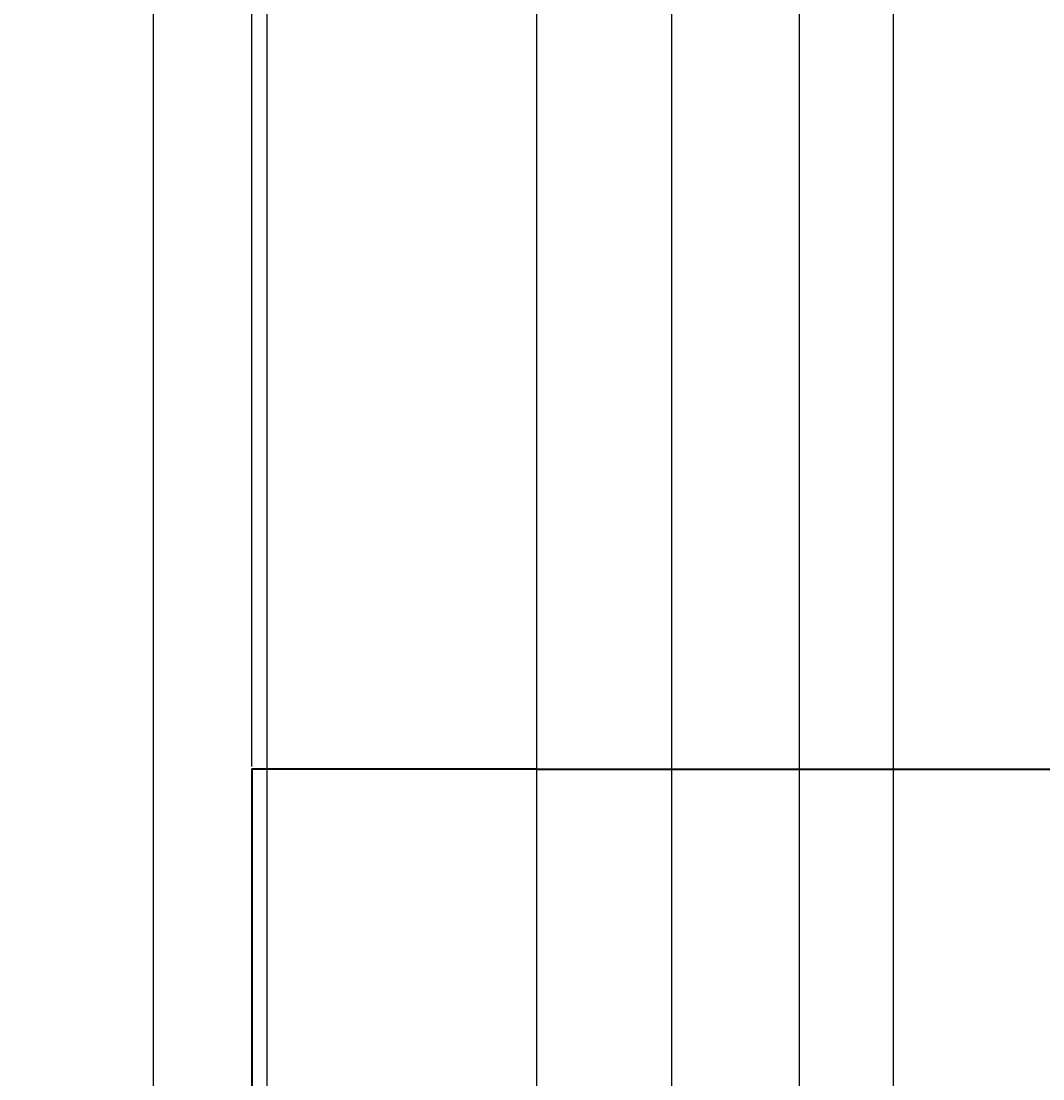
# Model space of a CAD drawing. Units: inches. Extents: x -6 to 289, y -8 to 323.
# Tile 79 of 107: x 104 to 126, y 252 to 276. Entities that reach past the tile are written whole.
import ezdxf

# ---------------------------------------------------------------- set-up
doc = ezdxf.new("R2010")
doc.units = ezdxf.units.IN
doc.header["$MEASUREMENT"] = 0
doc.layers.add('A-ANNO-DIMS', color=2, linetype='Continuous', lineweight=18)
doc.layers.add('A-ELEV', color=7, linetype='Continuous', lineweight=35)
doc.styles.get("Standard").update_dxf_attribs({"font": 'arial.ttf'})
doc.dimstyles.get("Standard").update_dxf_attribs({"dimtxt": 0.18, "dimasz": 0.18, "dimexe": 0.18, "dimexo": 0.0625, "dimgap": 0.09, "dimtad": 0, "dimtih": 1, "dimtoh": 1, "dimdec": 4, "dimzin": 0, "dimdsep": 46, "dimtxsty": 'Standard', "dimcen": 0.09, "dimadec": 0, "dimazin": 0, "dimtfac": 1, "dimtdec": 4, "dimtofl": 0, "dimtmove": 0, "dimatfit": 3, "dimfxl": 1, "dimtolj": 1, "dimtzin": 0, "dimarcsym": 0})

# ---------------------------------------------------------------- blocks, each defined once
blk = doc.blocks.new('*D10')
at = {"layer": 'A-ANNO-DIMS', "color": 0, "lineweight": -2, "transparency": 16777216}
for p, q in [((115.164, 307.351), (115.164, 322.969)), ((126.883, 226.717), (126.883, 322.969)), ((115.344, 322.789), (120.639, 322.789)), ((126.703, 322.789), (121.408, 322.789))]:
    blk.add_line(p, q, dxfattribs=at)
at = {"layer": 'A-ANNO-DIMS', "color": 0, "transparency": 16777216}
for points in [[(115.344, 322.819), (115.344, 322.759), (115.164, 322.789)], [(126.703, 322.819), (126.703, 322.759), (126.883, 322.789)]]:
    blk.add_solid(points, dxfattribs=at)
at = {"layer": 'Defpoints', "color": 0, "transparency": 16777216}
for p in [(126.883, 322.789), (115.164, 307.289), (126.883, 226.654)]:
    blk.add_point(p, dxfattribs=at)
at = {"layer": 'A-ANNO-DIMS', "color": 0, "transparency": 16777216, "insert": (121.024, 322.789), "char_height": 0.18, "attachment_point": 5}
blk.add_mtext('\\A1;11.72', dxfattribs=at)
blk = doc.blocks.new('*D27')
at = {"layer": 'A-ANNO-DIMS', "color": 0, "lineweight": -2, "transparency": 16777216}
for p, q in [((19.226, 307.289), (288.653, 307.289)), ((288.473, 307.109), (288.473, 277.471)), ((288.473, 247.469), (288.473, 277.107)), ((247.226, 247.289), (288.653, 247.289))]:
    blk.add_line(p, q, dxfattribs=at)
at = {"layer": 'A-ANNO-DIMS', "color": 0, "transparency": 16777216}
for points in [[(288.443, 307.109), (288.503, 307.109), (288.473, 307.289)], [(288.443, 247.469), (288.503, 247.469), (288.473, 247.289)]]:
    blk.add_solid(points, dxfattribs=at)
at = {"layer": 'Defpoints', "color": 0, "transparency": 16777216}
for p in [(19.164, 307.289), (288.473, 307.289), (247.164, 247.289)]:
    blk.add_point(p, dxfattribs=at)
at = {"layer": 'A-ANNO-DIMS', "color": 0, "transparency": 16777216, "insert": (288.473, 277.289), "char_height": 0.18, "attachment_point": 5}
blk.add_mtext('\\A1;60', dxfattribs=at)
blk = doc.blocks.new('*D58')
at = {"layer": 'A-ANNO-DIMS', "color": 0, "lineweight": -2, "transparency": 16777216}
for p, q in [((106.634, 68.495), (106.634, 322.969)), ((123.094, 68.495), (123.094, 322.969)), ((106.814, 322.789), (114.479, 322.789)), ((122.914, 322.789), (115.249, 322.789))]:
    blk.add_line(p, q, dxfattribs=at)
at = {"layer": 'A-ANNO-DIMS', "color": 0, "transparency": 16777216}
for points in [[(106.814, 322.819), (106.814, 322.759), (106.634, 322.789)], [(122.914, 322.819), (122.914, 322.759), (123.094, 322.789)]]:
    blk.add_solid(points, dxfattribs=at)
at = {"layer": 'Defpoints', "color": 0, "transparency": 16777216}
for p in [(123.094, 322.789), (106.634, 68.432), (123.094, 68.432)]:
    blk.add_point(p, dxfattribs=at)
at = {"layer": 'A-ANNO-DIMS', "color": 0, "transparency": 16777216, "insert": (114.864, 322.789), "char_height": 0.18, "attachment_point": 5}
blk.add_mtext('\\A1;16.46', dxfattribs=at)
blk = doc.blocks.new('*D73')
at = {"layer": 'A-ANNO-DIMS', "color": 0, "lineweight": -2, "transparency": 16777216}
for p, q in [((121.008, 51.148), (121.008, 322.969)), ((135.296, 51.148), (135.296, 322.969)), ((121.188, 322.789), (127.697, 322.789)), ((135.116, 322.789), (128.607, 322.789))]:
    blk.add_line(p, q, dxfattribs=at)
at = {"layer": 'A-ANNO-DIMS', "color": 0, "transparency": 16777216}
for points in [[(121.188, 322.819), (121.188, 322.759), (121.008, 322.789)], [(135.116, 322.819), (135.116, 322.759), (135.296, 322.789)]]:
    blk.add_solid(points, dxfattribs=at)
at = {"layer": 'Defpoints', "color": 0, "transparency": 16777216}
for p in [(135.296, 322.789), (121.008, 51.085), (135.296, 51.085)]:
    blk.add_point(p, dxfattribs=at)
at = {"layer": 'A-ANNO-DIMS', "color": 0, "transparency": 16777216, "insert": (128.152, 322.789), "char_height": 0.18, "attachment_point": 5}
blk.add_mtext('\\A1;14.288', dxfattribs=at)
blk = doc.blocks.new('*D92')
at = {"layer": 'A-ANNO-DIMS', "color": 0, "lineweight": -2, "transparency": 16777216}
for p, q in [((109.164, 127.351), (109.164, 322.969)), ((115.164, 162.411), (115.164, 322.969)), ((109.344, 322.789), (112.014, 322.789)), ((114.984, 322.789), (112.313, 322.789))]:
    blk.add_line(p, q, dxfattribs=at)
at = {"layer": 'A-ANNO-DIMS', "color": 0, "transparency": 16777216}
for points in [[(109.344, 322.819), (109.344, 322.759), (109.164, 322.789)], [(114.984, 322.819), (114.984, 322.759), (115.164, 322.789)]]:
    blk.add_solid(points, dxfattribs=at)
at = {"layer": 'Defpoints', "color": 0, "transparency": 16777216}
for p in [(115.164, 322.789), (115.164, 162.348), (109.164, 127.289)]:
    blk.add_point(p, dxfattribs=at)
at = {"layer": 'A-ANNO-DIMS', "color": 0, "transparency": 16777216, "insert": (112.164, 322.789), "char_height": 0.18, "attachment_point": 5}
blk.add_mtext('\\A1;6', dxfattribs=at)
blk = doc.blocks.new('*D93')
at = {"layer": 'A-ANNO-DIMS', "color": 0, "lineweight": -2, "transparency": 16777216}
for p, q in [((115.164, 162.411), (115.164, 322.969)), ((118.164, 159.411), (118.164, 322.969)), ((115.344, 322.789), (116.515, 322.789)), ((117.984, 322.789), (116.813, 322.789))]:
    blk.add_line(p, q, dxfattribs=at)
at = {"layer": 'A-ANNO-DIMS', "color": 0, "transparency": 16777216}
for points in [[(115.344, 322.819), (115.344, 322.759), (115.164, 322.789)], [(117.984, 322.819), (117.984, 322.759), (118.164, 322.789)]]:
    blk.add_solid(points, dxfattribs=at)
at = {"layer": 'Defpoints', "color": 0, "transparency": 16777216}
for p in [(118.164, 322.789), (115.164, 162.348), (118.164, 159.348)]:
    blk.add_point(p, dxfattribs=at)
at = {"layer": 'A-ANNO-DIMS', "color": 0, "transparency": 16777216, "insert": (116.664, 322.789), "char_height": 0.18, "attachment_point": 5}
blk.add_mtext('\\A1;3', dxfattribs=at)
blk = doc.blocks.new('*D94')
at = {"layer": 'A-ANNO-DIMS', "color": 0, "lineweight": -2, "transparency": 16777216}
for p, q in [((118.164, 159.411), (118.164, 322.969)), ((161.552, 159.411), (161.552, 322.969)), ((118.344, 322.789), (139.46, 322.789)), ((161.372, 322.789), (140.256, 322.789))]:
    blk.add_line(p, q, dxfattribs=at)
at = {"layer": 'A-ANNO-DIMS', "color": 0, "transparency": 16777216}
for points in [[(118.344, 322.819), (118.344, 322.759), (118.164, 322.789)], [(161.372, 322.819), (161.372, 322.759), (161.552, 322.789)]]:
    blk.add_solid(points, dxfattribs=at)
at = {"layer": 'Defpoints', "color": 0, "transparency": 16777216}
for p in [(161.552, 322.789), (118.164, 159.348), (161.552, 159.348)]:
    blk.add_point(p, dxfattribs=at)
at = {"layer": 'A-ANNO-DIMS', "color": 0, "transparency": 16777216, "insert": (139.858, 322.789), "char_height": 0.18, "attachment_point": 5}
blk.add_mtext('\\A1;43.39', dxfattribs=at)
blk = doc.blocks.new('*D105')
at = {"layer": 'A-ANNO-DIMS', "color": 0, "lineweight": -2, "transparency": 16777216}
for p, q in [((108.823, 259.351), (108.823, 322.969)), ((115.164, 277.105), (115.164, 322.969)), ((109.003, 322.789), (111.616, 322.789)), ((114.984, 322.789), (112.37, 322.789))]:
    blk.add_line(p, q, dxfattribs=at)
at = {"layer": 'A-ANNO-DIMS', "color": 0, "transparency": 16777216}
for points in [[(109.003, 322.819), (109.003, 322.759), (108.823, 322.789)], [(114.984, 322.819), (114.984, 322.759), (115.164, 322.789)]]:
    blk.add_solid(points, dxfattribs=at)
at = {"layer": 'Defpoints', "color": 0, "transparency": 16777216}
for p in [(115.164, 322.789), (115.164, 277.043), (108.823, 259.289)]:
    blk.add_point(p, dxfattribs=at)
at = {"layer": 'A-ANNO-DIMS', "color": 0, "transparency": 16777216, "insert": (111.993, 322.789), "char_height": 0.18, "attachment_point": 5}
blk.add_mtext('\\A1;6.341', dxfattribs=at)

msp = doc.modelspace()

# ---------------------------------------------------------------- linework, layer by layer
at = {"layer": 'A-ELEV'}
msp.add_line((115.1638, 259.2888), (271.1638, 259.2888), dxfattribs=at)
msp.add_lwpolyline([(115.1638, 259.2888), (108.8227, 259.2888), (108.8227, 247.2888), (115.1638, 247.2888)], dxfattribs=at)

# ---------------------------------------------------------------- dimensions: what is measured, and where the dimension line sits
at = {"layer": 'A-ANNO-DIMS'}
for base, p1, p2, override, picture, middle in [((123.094, 322.7888), (106.634, 68.4322), (123.094, 68.4322), {"dimdec": 2, "dimlfac": 1, "dimrnd": 0, "dimzin": 0, "dimdsep": 46, "dimlunit": 2}, '*D58', (114.864, 322.7888)), ((115.1638, 322.7888), (108.8227, 259.2888), (115.1638, 277.0427), {"dimdec": 3, "dimlfac": 1, "dimrnd": 0, "dimzin": 0, "dimdsep": 46, "dimlunit": 2}, '*D105', (111.9933, 322.7888)), ((115.1638, 322.7888), (109.1638, 127.2888), (115.1638, 162.3484), {"dimdec": 0, "dimlfac": 1, "dimrnd": 0, "dimzin": 0, "dimdsep": 46, "dimlunit": 2}, '*D92', (112.1638, 322.7888)), ((126.8835, 322.7888), (115.1638, 307.2888), (126.8835, 226.654), {"dimdec": 2, "dimlfac": 1, "dimrnd": 0, "dimzin": 0, "dimdsep": 46, "dimlunit": 2}, '*D10', (121.0236, 322.7888)), ((118.1638, 322.7888), (115.1638, 162.3484), (118.1638, 159.3484), {"dimdec": 0, "dimlfac": 1, "dimrnd": 0, "dimzin": 0, "dimdsep": 46, "dimlunit": 2}, '*D93', (116.6638, 322.7888)), ((161.5522, 322.7888), (118.1638, 159.3484), (161.5522, 159.3484), {"dimdec": 2, "dimlfac": 1, "dimrnd": 0, "dimzin": 0, "dimdsep": 46, "dimlunit": 2}, '*D94', (139.858, 322.7888)), ((135.296, 322.7888), (121.008, 51.0851), (135.296, 51.0851), {"dimdec": 3, "dimlfac": 1, "dimrnd": 0, "dimzin": 0, "dimdsep": 46, "dimlunit": 2}, '*D73', (128.152, 322.7888))]:
    dim = msp.add_linear_dim(base=base, p1=p1, p2=p2, dimstyle='Standard', override=override, dxfattribs=at)
    dim.commit()
    dim.dimension.update_dxf_attribs({"geometry": picture, "text_midpoint": middle})
dim = msp.add_linear_dim(base=(288.4733, 307.2888), p1=(247.1638, 247.2888), p2=(19.1638, 307.2888), angle=90, dimstyle='Standard', override={"dimdec": 0, "dimlfac": 1, "dimrnd": 0, "dimzin": 0, "dimdsep": 46, "dimlunit": 2}, dxfattribs=at)
dim.commit()
dim.dimension.update_dxf_attribs({"geometry": '*D27', "text_midpoint": (288.4733, 277.2888)})

doc.saveas('drawing.dxf')
